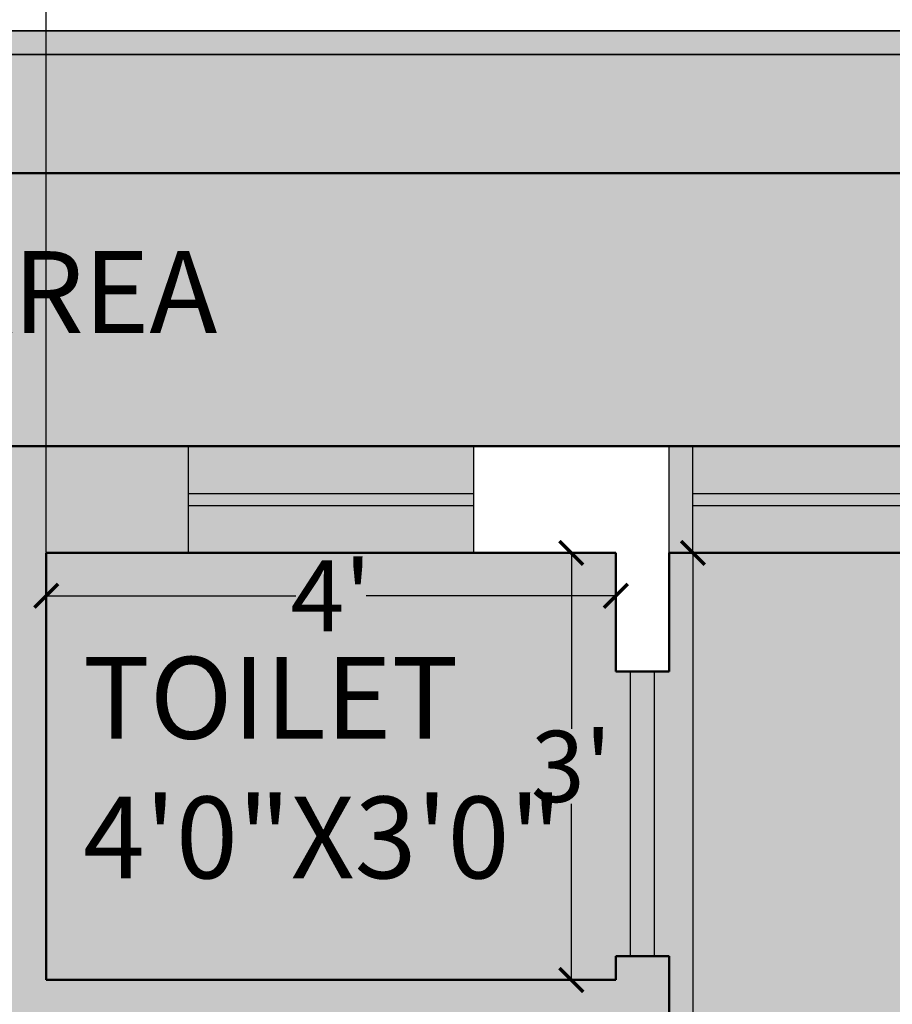
# Model space of a CAD drawing. Units: inches. Extents: x 528 to 2620, y -1066 to 798.
# Tile 17 of 41: x 776 to 850, y 672 to 755. Entities that reach past the tile are written whole.
import ezdxf

# ---------------------------------------------------------------- set-up
doc = ezdxf.new("R2010")
doc.units = ezdxf.units.IN
doc.header["$MEASUREMENT"] = 0
for name, color, linetype, lineweight in [('A-ANNO-DIMS', 2, 'Continuous', 18), ('A-AREA-IDEN', 7, 'Continuous', 18), ('A-Door', 2, 'Continuous', 25), ('A-GLAZ', 3, 'Continuous', 25), ('A-WALL', 7, 'Continuous', 50), ('A-WALL-PATT', 8, 'Continuous', 13), ('C-PROP', 5, 'Continuous', 35)]:
    doc.layers.add(name, color=color, linetype=linetype, lineweight=lineweight)
doc.styles.get("Standard").update_dxf_attribs({"font": 'arial.ttf'})
doc.dimstyles.get("Standard").update_dxf_attribs({"dimtxt": 6, "dimasz": 2, "dimexe": 0.18, "dimexo": 0.0625, "dimgap": 0.09, "dimtad": 0, "dimtih": 1, "dimtoh": 1, "dimdec": 1, "dimzin": 0, "dimdsep": 46, "dimlunit": 3, "dimtxsty": 'Standard', "dimblk": 'ARCHTICK', "dimcen": 0.09, "dimadec": 0, "dimazin": 0, "dimtfac": 1, "dimtdec": 1, "dimtofl": 0, "dimtmove": 0, "dimatfit": 3, "dimfxl": 1, "dimtolj": 1, "dimtzin": 0, "dimarcsym": 0})

# ---------------------------------------------------------------- blocks, each defined once
blk = doc.blocks.new('_ArchTick')
at = {"color": 0, "linetype": 'ByBlock', "const_width": 0.15}
blk.add_lwpolyline([(-0.5, -0.5), (0.5, 0.5)], dxfattribs=at)
blk = doc.blocks.new('*D11')
at = {"layer": 'A-ANNO-DIMS', "color": 0, "lineweight": -2, "transparency": 16777216}
for p, q in [((584.059, 753.985), (584.059, 794.007)), ((584.059, 793.827), (758.88, 793.827)), ((944.059, 793.827), (769.239, 793.827)), ((944.059, 753.985), (944.059, 794.007))]:
    blk.add_line(p, q, dxfattribs=at)
at = {"layer": 'Defpoints', "color": 0, "transparency": 16777216}
for p in [(944.059, 793.827), (584.059, 753.922), (944.059, 753.922)]:
    blk.add_point(p, dxfattribs=at)
at = {"layer": 'A-ANNO-DIMS', "color": 0, "lineweight": -2, "transparency": 16777216, "xscale": 2, "yscale": 2, "zscale": 2, "rotation": 180}
blk.add_blockref('_ArchTick', (584.059, 793.827), dxfattribs=at)
at = {"layer": 'A-ANNO-DIMS', "color": 0, "lineweight": -2, "transparency": 16777216, "xscale": 2, "yscale": 2, "zscale": 2}
blk.add_blockref('_ArchTick', (944.059, 793.827), dxfattribs=at)
at = {"layer": 'A-ANNO-DIMS', "color": 0, "transparency": 16777216, "insert": (764.059, 793.827), "char_height": 6, "attachment_point": 5}
blk.add_mtext("\\A1;30'", dxfattribs=at)
blk = doc.blocks.new('*D28')
at = {"layer": 'A-ANNO-DIMS', "color": 0, "lineweight": -2, "transparency": 16777216}
for p, q in [((833.059, 709.922), (833.059, 620.826)), ((833.122, 709.922), (833.239, 709.922)), ((833.059, 525.422), (833.059, 614.519)), ((833.102, 525.422), (832.879, 525.422))]:
    blk.add_line(p, q, dxfattribs=at)
at = {"layer": 'Defpoints', "color": 0, "transparency": 16777216}
for p in [(833.059, 709.922), (833.059, 709.922), (833.164, 525.422)]:
    blk.add_point(p, dxfattribs=at)
at = {"layer": 'A-ANNO-DIMS', "color": 0, "lineweight": -2, "transparency": 16777216, "xscale": 2, "yscale": 2, "zscale": 2}
for p, rotation in [((833.059, 709.922), 90), ((833.059, 525.422), 270)]:
    blk.add_blockref('_ArchTick', p, dxfattribs=dict(at, rotation=rotation))
at = {"layer": 'A-ANNO-DIMS', "color": 0, "transparency": 16777216, "insert": (833.059, 617.672), "char_height": 6, "attachment_point": 5}
blk.add_mtext('\\A1;15\'-4.5"', dxfattribs=at)
blk = doc.blocks.new('*D29')
at = {"layer": 'A-ANNO-DIMS', "color": 0, "lineweight": -2, "transparency": 16777216}
for p, q in [((822.67, 709.922), (822.995, 709.922)), ((822.815, 709.922), (822.815, 695.078)), ((822.815, 673.922), (822.815, 688.767)), ((822.67, 673.922), (822.995, 673.922))]:
    blk.add_line(p, q, dxfattribs=at)
at = {"layer": 'Defpoints', "color": 0, "transparency": 16777216}
for p in [(822.608, 709.922), (822.608, 673.922), (822.815, 673.922)]:
    blk.add_point(p, dxfattribs=at)
at = {"layer": 'A-ANNO-DIMS', "color": 0, "lineweight": -2, "transparency": 16777216, "xscale": 2, "yscale": 2, "zscale": 2}
for p, rotation in [((822.815, 709.922), 90), ((822.815, 673.922), 270)]:
    blk.add_blockref('_ArchTick', p, dxfattribs=dict(at, rotation=rotation))
at = {"layer": 'A-ANNO-DIMS', "color": 0, "transparency": 16777216, "insert": (822.815, 691.922), "char_height": 6, "attachment_point": 5}
blk.add_mtext("\\A1;3'", dxfattribs=at)
blk = doc.blocks.new('*D30')
at = {"layer": 'A-ANNO-DIMS', "color": 0, "lineweight": -2, "transparency": 16777216}
for p, q in [((778.559, 706.368), (778.559, 706.486)), ((778.559, 706.306), (799.588, 706.306)), ((826.559, 706.306), (805.531, 706.306)), ((826.559, 706.368), (826.559, 706.486))]:
    blk.add_line(p, q, dxfattribs=at)
at = {"layer": 'Defpoints', "color": 0, "transparency": 16777216}
for p in [(778.559, 706.306), (778.559, 706.306), (826.559, 706.306)]:
    blk.add_point(p, dxfattribs=at)
at = {"layer": 'A-ANNO-DIMS', "color": 0, "lineweight": -2, "transparency": 16777216, "xscale": 2, "yscale": 2, "zscale": 2, "rotation": 180}
blk.add_blockref('_ArchTick', (778.559, 706.306), dxfattribs=at)
at = {"layer": 'A-ANNO-DIMS', "color": 0, "lineweight": -2, "transparency": 16777216, "xscale": 2, "yscale": 2, "zscale": 2}
blk.add_blockref('_ArchTick', (826.559, 706.306), dxfattribs=at)
at = {"layer": 'A-ANNO-DIMS', "color": 0, "transparency": 16777216, "insert": (802.559, 706.306), "char_height": 6, "attachment_point": 5}
blk.add_mtext("\\A1;4'", dxfattribs=at)
blk = doc.blocks.new('WIN-1200')
for p, q in [((677.559, 718.922), (725.559, 718.922)), ((677.559, 709.922), (677.559, 718.922)), ((679.559, 709.922), (679.559, 718.922)), ((723.559, 718.922), (723.559, 709.922)), ((725.559, 718.922), (725.559, 709.922)), ((679.559, 714.922), (723.559, 714.922)), ((679.559, 713.922), (723.559, 713.922)), ((725.559, 709.922), (677.559, 709.922))]:
    blk.add_line(p, q)
blk = doc.blocks.new('WIN-600')
for p, q in [((790.559, 714.922), (814.559, 714.922)), ((790.559, 713.922), (814.559, 713.922))]:
    blk.add_line(p, q)
blk.add_lwpolyline([(790.559, 718.922), (814.559, 718.922), (814.559, 709.922), (790.559, 709.922)], close=True)
blk = doc.blocks.new('*D56')
at = {"layer": 'A-ANNO-DIMS', "color": 0, "lineweight": -2, "transparency": 16777216}
for p, q in [((774.059, 709.985), (774.059, 788.102)), ((774.059, 787.922), (778.559, 787.922)), ((778.559, 709.985), (778.559, 788.102)), ((778.559, 787.922), (780.559, 787.922))]:
    blk.add_line(p, q, dxfattribs=at)
at = {"layer": 'Defpoints', "color": 0, "transparency": 16777216}
for p in [(778.559, 787.922), (774.059, 709.922), (778.559, 709.922)]:
    blk.add_point(p, dxfattribs=at)
at = {"layer": 'A-ANNO-DIMS', "color": 0, "lineweight": -2, "transparency": 16777216, "xscale": 2, "yscale": 2, "zscale": 2, "rotation": 180}
blk.add_blockref('_ArchTick', (774.059, 787.922), dxfattribs=at)
at = {"layer": 'A-ANNO-DIMS', "color": 0, "lineweight": -2, "transparency": 16777216, "xscale": 2, "yscale": 2, "zscale": 2}
blk.add_blockref('_ArchTick', (778.559, 787.922), dxfattribs=at)
at = {"layer": 'A-ANNO-DIMS', "color": 0, "transparency": 16777216, "insert": (795.615, 787.922), "char_height": 6, "attachment_point": 5}
blk.add_mtext('\\A1;0\'-4 1/2"', dxfattribs=at)

msp = doc.modelspace()

# ---------------------------------------------------------------- hatches: boundary and pattern name
at = {"layer": 'A-Door', "transparency": 33554521}
h = msp.add_hatch(color=256, dxfattribs=at)
h.dxf.hatch_style = 1
h.paths.add_polyline_path([(829.809, 699.922), (827.809, 699.922), (827.809, 675.922), (829.809, 675.922)])
at = {"layer": 'A-WALL-PATT', "transparency": 33554687}
h = msp.add_hatch(color=256, dxfattribs=at)
h.dxf.hatch_style = 1
h.paths.add_polyline_path([(944.059, 753.922), (584.059, 753.922), (584.059, 208.922), (608.059, 208.922), (608.059, 210.922), (586.059, 210.922), (586.059, 751.922), (942.059, 751.922), (942.059, 210.922), (728.059, 210.922), (728.059, 208.922), (944.059, 208.922)])
h = msp.add_hatch(color=256, dxfattribs=at)
h.dxf.hatch_style = 1
h.paths.add_polyline_path([(942.059, 751.922), (586.059, 751.922), (586.059, 210.922), (608.059, 210.922), (608.059, 220.922), (596.059, 220.922), (596.059, 741.922), (932.059, 741.922), (932.059, 220.922), (770.059, 220.922), (728.059, 220.922), (728.059, 210.922), (942.059, 210.922)])
at = {"layer": 'A-WALL-PATT', "transparency": 33554475}
h = msp.add_hatch(color=256, dxfattribs=at)
h.dxf.hatch_style = 1
h.paths.add_polyline_path([(620.059, 718.922), (908.059, 718.922), (908.059, 268.922), (770.059, 268.922), (770.059, 220.922), (932.059, 220.922), (932.059, 741.922), (596.059, 741.922), (596.059, 391.422), (620.059, 391.422)])
at = {"layer": 'A-WALL-PATT', "transparency": 33554687}
h = msp.add_hatch(color=256, dxfattribs=at)
h.dxf.hatch_style = 1
h.paths.add_polyline_path([(861.059, 273.922), (817.059, 273.922), (817.059, 272.922), (861.059, 272.922)])
h.paths.add_polyline_path([(817.059, 277.922), (815.059, 277.922), (815.059, 268.922), (817.059, 268.922)])
h.paths.add_polyline_path([(908.059, 397.922), (899.059, 397.922), (899.059, 395.922), (908.059, 395.922)])
h.paths.add_polyline_path([(908.059, 443.922), (899.059, 443.922), (899.059, 441.922), (908.059, 441.922)])
h.paths.add_polyline_path([(904.059, 441.922), (903.059, 441.922), (903.059, 397.922), (904.059, 397.922)])
h.paths.add_polyline_path([(625.059, 561.422), (624.059, 561.422), (624.059, 537.422), (625.059, 537.422)])
h.paths.add_polyline_path([(648.747, 334.444), (720.045, 334.444), (720.045, 344.998), (648.747, 344.998)], flags=9)
h.paths.add_polyline_path([(819.733, 323.153), (880.328, 323.153), (880.328, 333.708), (819.733, 333.708)], flags=9)
h.paths.add_polyline_path([(779.898, 680.607), (821.764, 680.607), (821.764, 691.169), (779.898, 691.169)], flags=9)
h.paths.add_polyline_path([(779.876, 692.362), (817.138, 692.362), (817.138, 703.058), (779.876, 703.058)], flags=9)
h.paths.add_polyline_path([(799.994, 453.884), (860.589, 453.884), (860.589, 464.439), (799.994, 464.439)], flags=9)
h.paths.add_polyline_path([(650.866, 539.397), (708.781, 539.397), (708.781, 549.952), (650.866, 549.952)], flags=9)
h.paths.add_polyline_path([(788.504, 612.01), (849.099, 612.01), (849.099, 622.565), (788.504, 622.565)], flags=9)
h.paths.add_polyline_path([(639.539, 648.31), (700.134, 648.31), (700.134, 658.865), (639.539, 658.865)], flags=9)
h.paths.add_polyline_path([(648.913, 346.09), (747.706, 346.09), (747.706, 356.778), (648.913, 356.778)], flags=9)
h.paths.add_polyline_path([(676.857, 450.66), (746.735, 450.66), (746.735, 461.355), (676.857, 461.355)], flags=9)
h.paths.add_polyline_path([(819.711, 334.947), (865.526, 334.947), (865.526, 345.636), (819.711, 345.636)], flags=9)
h.paths.add_polyline_path([(806.298, 467.745), (874.047, 467.745), (874.047, 478.441), (806.298, 478.441)], flags=9)
h.paths.add_polyline_path([(653.235, 552.284), (690.497, 552.284), (690.497, 562.979), (653.235, 562.979)], flags=9)
h.paths.add_polyline_path([(789.903, 623.407), (843.208, 623.407), (843.208, 634.103), (789.903, 634.103)], flags=9)
h.paths.add_polyline_path([(639.773, 662.103), (693.077, 662.103), (693.077, 672.798), (639.773, 672.798)], flags=9)
h.paths.add_polyline_path([(801.587, 242.914), (846.334, 242.914), (846.334, 253.603), (801.587, 253.603)], flags=9)
h.paths.add_polyline_path([(925.362, 593.982), (925.362, 674.057), (914.673, 674.057), (914.673, 593.982)], flags=9)
h.paths.add_polyline_path([(612.559, 593.982), (612.559, 674.057), (601.871, 674.057), (601.871, 593.982)], flags=9)
h.paths.add_polyline_path([(723.31, 726.564), (803.385, 726.564), (803.385, 737.252), (723.31, 737.252)], flags=9)
at = {"layer": 'A-WALL-PATT', "transparency": 33554521}
h = msp.add_hatch(color=256, dxfattribs=at)
h.dxf.hatch_style = 1
h.paths.add_polyline_path([(629.059, 709.922), (677.559, 709.922), (677.559, 718.922), (620.059, 718.922), (620.059, 667.922), (629.059, 667.922)])
h.paths.add_polyline_path([(790.559, 718.922), (725.559, 718.922), (725.559, 709.922), (774.059, 709.922), (774.059, 577.922), (768.481, 577.922), (768.559, 573.422), (774.059, 573.422), (774.059, 567.422), (778.559, 567.422), (778.559, 669.422), (831.059, 669.422), (831.059, 675.922), (826.559, 675.922), (826.559, 673.922), (778.559, 673.922), (778.559, 709.922), (790.559, 709.922)])
h.paths.add_polyline_path([(908.059, 718.922), (879.059, 718.922), (879.059, 709.922), (899.059, 709.922), (899.059, 641.672), (908.059, 641.672)])
h.paths.add_polyline_path([(629.059, 619.922), (620.059, 619.922), (620.059, 561.422), (629.059, 561.422), (629.059, 573.422), (724.059, 573.422), (724.059, 569.422), (728.559, 569.422), (728.559, 577.922), (629.059, 577.922)])
h.paths.add_polyline_path([(779.059, 391.422), (779.059, 400.422), (770.059, 400.422), (764.059, 400.422), (764.059, 397.422), (764.059, 391.422), (770.059, 391.422), (770.059, 268.922), (815.059, 268.922), (815.059, 277.922), (779.059, 277.922), (779.059, 359.767)])
h.paths.add_polyline_path([(908.059, 395.922), (899.059, 395.922), (851.059, 395.922), (851.059, 391.422), (899.059, 391.422), (899.059, 277.922), (863.059, 277.922), (863.059, 268.922), (908.059, 268.922)])
h.paths.add_polyline_path([(908.059, 593.672), (899.059, 593.672), (899.059, 525.422), (778.559, 525.422), (778.559, 527.172), (774.059, 527.172), (774.059, 520.922), (899.059, 520.922), (899.059, 443.922), (908.059, 443.922)])
h.paths.add_polyline_path([(629.059, 520.922), (728.559, 520.922), (728.559, 545.422), (724.059, 545.422), (724.059, 525.422), (629.059, 525.422), (629.059, 537.422), (620.059, 537.422), (620.059, 484.672), (629.059, 484.672)])
h.paths.add_polyline_path([(629.059, 436.672), (620.059, 436.672), (620.059, 391.422), (648.559, 391.422), (648.559, 400.422), (629.059, 400.422)])
h.paths.add_polyline_path([(716.059, 397.422), (716.059, 400.422), (696.559, 400.422), (696.559, 391.422), (716.059, 391.422)])
at = {"layer": 'A-WALL-PATT', "transparency": 33554681}
h = msp.add_hatch(color=256, dxfattribs=at)
h.dxf.hatch_style = 1
h.paths.add_polyline_path([(629.059, 665.922), (625.059, 665.922), (625.059, 621.922), (629.059, 621.922)])
h.paths.add_polyline_path([(624.059, 665.922), (620.059, 665.922), (620.059, 621.922), (624.059, 621.922)])
h.paths.add_polyline_path([(723.559, 713.922), (679.559, 713.922), (679.559, 709.922), (723.559, 709.922)])
h.paths.add_polyline_path([(723.559, 718.922), (679.559, 718.922), (679.559, 714.922), (723.559, 714.922)])
h.paths.add_polyline_path([(814.559, 713.922), (790.559, 713.922), (790.559, 709.922), (814.559, 709.922)])
h.paths.add_polyline_path([(814.559, 718.922), (790.559, 718.922), (790.559, 714.922), (814.559, 714.922)])
h.paths.add_polyline_path([(877.059, 713.922), (833.059, 713.922), (833.059, 709.922), (877.059, 709.922)])
h.paths.add_polyline_path([(877.059, 718.922), (833.059, 718.922), (833.059, 714.922), (877.059, 714.922)])
h.paths.add_polyline_path([(908.059, 639.672), (904.059, 639.672), (904.059, 595.672), (908.059, 595.672)])
h.paths.add_polyline_path([(903.059, 639.672), (899.059, 639.672), (899.059, 595.672), (903.059, 595.672)])
h.paths.add_polyline_path([(908.059, 441.922), (904.059, 441.922), (904.059, 397.922), (908.059, 397.922)])
h.paths.add_polyline_path([(903.059, 441.922), (899.059, 441.922), (899.059, 397.922), (903.059, 397.922)])
h.paths.add_polyline_path([(861.059, 272.922), (817.059, 272.922), (817.059, 268.922), (861.059, 268.922)])
h.paths.add_polyline_path([(861.059, 277.922), (817.059, 277.922), (817.059, 273.922), (861.059, 273.922)])
h.paths.add_polyline_path([(694.559, 395.422), (650.559, 395.422), (650.559, 391.422), (694.559, 391.422)])
h.paths.add_polyline_path([(694.559, 400.422), (650.559, 400.422), (650.559, 396.422), (694.559, 396.422)])
h.paths.add_polyline_path([(629.059, 482.672), (625.059, 482.672), (625.059, 438.672), (629.059, 438.672)])
h.paths.add_polyline_path([(624.059, 482.672), (620.059, 482.672), (620.059, 438.672), (624.059, 438.672)])
h.paths.add_polyline_path([(629.059, 561.422), (625.059, 561.422), (625.059, 537.422), (629.059, 537.422)])
h.paths.add_polyline_path([(624.059, 561.422), (620.059, 561.422), (620.059, 537.422), (624.059, 537.422)])
h = msp.add_hatch(color=256, dxfattribs=at)
h.dxf.hatch_style = 1
h.paths.add_polyline_path([(625.059, 665.922), (624.059, 665.922), (624.059, 621.922), (625.059, 621.922)])
h.paths.add_polyline_path([(629.059, 667.922), (620.059, 667.922), (620.059, 665.922), (629.059, 665.922)])
h.paths.add_polyline_path([(629.059, 621.922), (620.059, 621.922), (620.059, 619.922), (629.059, 619.922)])
h.paths.add_polyline_path([(723.559, 714.922), (679.559, 714.922), (679.559, 713.922), (723.559, 713.922)])
h.paths.add_polyline_path([(725.559, 718.922), (723.559, 718.922), (723.559, 709.922), (725.559, 709.922)])
h.paths.add_polyline_path([(679.559, 718.922), (677.559, 718.922), (677.559, 709.922), (679.559, 709.922)])
h.paths.add_polyline_path([(814.559, 714.922), (790.559, 714.922), (790.559, 713.922), (814.559, 713.922)])
h.paths.add_polyline_path([(877.059, 714.922), (833.059, 714.922), (833.059, 713.922), (877.059, 713.922)])
h.paths.add_polyline_path([(879.059, 718.922), (877.059, 718.922), (877.059, 709.922), (879.059, 709.922)])
h.paths.add_polyline_path([(833.059, 718.922), (831.059, 718.922), (831.059, 709.922), (833.059, 709.922)])
h.paths.add_polyline_path([(650.559, 400.422), (648.559, 400.422), (648.559, 391.422), (650.559, 391.422)])
h.paths.add_polyline_path([(694.559, 396.422), (650.559, 396.422), (650.559, 395.422), (694.559, 395.422)])
h.paths.add_polyline_path([(696.559, 400.422), (694.559, 400.422), (694.559, 391.422), (696.559, 391.422)])
h.paths.add_polyline_path([(629.059, 438.672), (620.059, 438.672), (620.059, 436.672), (629.059, 436.672)])
h.paths.add_polyline_path([(629.059, 484.672), (620.059, 484.672), (620.059, 482.672), (629.059, 482.672)])
h.paths.add_polyline_path([(625.059, 482.672), (624.059, 482.672), (624.059, 438.672), (625.059, 438.672)])
at = {"layer": 'A-WALL-PATT', "transparency": 33554590}
h = msp.add_hatch(color=256, dxfattribs=at)
h.dxf.hatch_style = 1
h.paths.add_polyline_path([(774.059, 709.922), (629.059, 709.922), (629.059, 577.922), (728.559, 577.922), (728.559, 579.422), (728.559, 619.422), (730.309, 619.422), (730.309, 619.384, -0.401453), (768.559, 579.422), (768.559, 577.922), (774.059, 577.922)])
h.paths.add_polyline_path([(723.896, 686.058), (723.968, 686.064), (723.828, 686.128)], flags=0)
h.paths.add_polyline_path([(722.785, 642.699), (722.893, 642.756), (722.893, 684.992), (722.647, 685.244), (722.647, 685.82), (723.079, 686.262), (723.533, 686.262), (723.968, 686.064), (724.739, 686.128), (770.696, 686.128), (770.78, 686.14), (771.126, 686.266), (771.694, 686.094), (771.94, 685.478), (771.67, 684.904), (771.582, 684.871), (771.582, 642.782), (771.878, 642.514), (771.878, 641.921), (771.511, 641.462), (770.855, 641.462), (770.401, 641.833), (770.401, 641.551), (724.739, 641.551), (723.991, 641.705), (723.443, 641.414), (722.879, 641.585), (722.597, 642.142)], flags=16)
h.paths.add_polyline_path([(723.994, 641.704), (723.994, 641.707), (723.991, 641.705)], flags=0)
h.paths.add_polyline_path([(722.893, 642.732), (722.893, 684.992), (722.647, 685.244), (722.647, 685.82), (723.079, 686.262), (723.287, 686.262), (722.991, 686.172), (722.794, 685.971), (722.647, 685.68), (722.647, 685.434), (722.745, 685.143), (722.942, 684.942), (723.238, 684.807), (723.484, 684.807), (723.779, 684.897), (723.976, 685.098), (724.174, 685.488), (724.124, 685.635), (724.124, 685.249), (723.631, 684.746), (723.631, 642.961), (724.124, 642.514), (724.124, 641.887), (723.656, 641.462), (723.079, 641.462), (722.647, 641.904), (722.647, 642.48)], flags=0)
h.paths.add_polyline_path([(722.647, 642.29), (722.647, 642.044), (722.794, 641.753), (723.079, 641.462), (723.287, 641.462), (722.879, 641.585), (722.597, 642.142)], flags=0)
h.paths.add_polyline_path([(770.745, 686.128), (770.58, 686.128), (770.551, 686.057)], flags=0)
h.paths.add_polyline_path([(743.299, 645.288), (753.227, 659.398), (748.69, 663.75), (753.234, 668.538), (743.299, 682.458), (743.791, 682.592), (744.136, 682.681), (744.53, 682.928), (744.628, 683.084), (745.017, 683.327), (744.53, 684.069), (744.776, 684.158), (744.874, 684.315), (745.514, 684.404), (746.081, 684.651), (746.474, 684.651), (746.819, 684.807), (747.459, 685.031), (747.705, 685.143), (748.198, 685.277), (748.394, 685.523), (748.862, 685.523), (749.994, 686.128), (753.488, 676.03), (757.379, 680.153), (757.791, 679.758), (758.044, 680.645), (758.29, 681.227), (758.29, 682.055), (758.019, 682.592), (757.871, 683.174), (757.822, 683.778), (758.388, 684.069), (758.979, 684.203), (759.619, 684.158), (760.21, 683.957), (760.751, 683.666), (761.859, 683.666), (762.401, 683.957), (762.991, 684.114), (763.631, 684.114), (764.198, 683.957), (764.739, 683.666), (766.118, 683.666), (766.659, 683.957), (767.25, 684.158), (767.865, 684.203), (768.456, 684.069), (769.047, 683.778), (768.998, 683.174), (768.85, 682.592), (768.554, 682.055), (768.554, 681.227), (768.801, 680.645), (769.092, 679.75), (768.948, 678.832), (768.801, 678.228), (768.554, 677.646), (768.554, 676.818), (768.801, 676.237), (769.092, 675.341), (768.948, 674.424), (768.801, 673.82), (768.554, 673.283), (768.554, 672.41), (768.801, 671.873), (768.998, 671.291), (769.047, 670.642), (768.948, 670.016), (768.801, 669.411), (768.554, 668.874), (768.554, 668.002), (768.974, 667.239), (769.047, 666.279), (769.047, 665.563), (768.456, 665.316), (767.865, 665.16), (767.25, 665.16), (766.659, 665.361), (766.118, 665.697), (764.739, 665.697), (763.945, 665.204), (762.991, 665.204), (762.401, 665.361), (761.859, 665.697), (761.005, 665.697), (762.696, 664.086), (760.741, 662.027), (761.859, 662.027), (762.401, 662.318), (763.342, 662.548), (764.247, 662.318), (764.788, 662.027), (766.118, 662.027), (766.659, 662.318), (767.25, 662.519), (767.865, 662.564), (768.505, 662.43), (769.047, 662.116), (769.047, 661.4), (769.047, 660.796), (768.85, 660.214), (768.554, 659.677), (768.554, 658.849), (768.85, 658.267), (768.998, 657.663), (769.069, 656.749), (768.85, 655.851), (768.554, 655.269), (768.554, 654.441), (768.85, 653.859), (769.069, 652.961), (768.998, 652.046), (768.85, 651.442), (768.554, 650.905), (768.554, 650.032), (768.85, 649.495), (768.998, 648.914), (769.047, 648.265), (768.998, 647.638), (768.85, 647.034), (768.554, 646.497), (768.554, 645.624), (768.85, 645.087), (769.047, 644.55), (769.047, 643.901), (768.505, 643.655), (767.865, 643.521), (767.25, 643.521), (766.659, 643.722), (766.118, 644.058), (764.788, 644.058), (764.247, 643.722), (763.342, 643.492), (762.401, 643.722), (761.859, 644.058), (760.801, 644.058), (760.259, 643.722), (759.668, 643.521), (759.028, 643.521), (758.388, 643.655), (757.871, 643.901), (757.871, 644.55), (758.044, 645.087), (758.339, 645.624), (758.339, 646.497), (758.044, 647.034), (757.921, 647.638), (757.866, 648.059), (757.379, 647.593), (753.422, 651.773), (749.994, 641.618), (749.502, 641.708), (749.354, 641.954), (748.542, 642.446), (747.311, 642.939), (746.652, 642.939), (746.327, 643.185), (745.514, 643.565), (744.53, 643.655), (745.011, 644.4), (744.628, 644.639), (744.136, 644.886), (743.791, 645.132)], flags=0)
h.paths.add_polyline_path([(755.656, 654.933), (756.542, 654.687), (757.527, 654.329), (756.641, 654.575)], flags=0)
h.paths.add_polyline_path([(758.339, 649.204), (758.339, 648.712), (758.585, 644.304), (758.585, 648.802)], flags=0)
h.paths.add_polyline_path([(758.339, 649.294), (758.093, 649.697), (758.359, 649.165)], flags=0)
h.paths.add_polyline_path([(755.656, 672.79), (756.493, 673.037), (757.358, 673.351), (757.353, 673.358), (756.641, 673.149)], flags=0)
h.paths.add_polyline_path([(760.264, 639.641), (771.408, 639.641), (771.408, 624.039), (760.264, 624.039)], flags=16)
h.paths.add_polyline_path([(761.378, 638.526), (770.294, 638.526), (770.294, 625.153), (761.378, 625.153)], flags=0)
edge = h.paths.add_edge_path(flags=0)
edge.add_ellipse((765.836, 631.84), major_axis=(-2.245, 2.245), ratio=1, start_angle=-45, end_angle=45, ccw=False)
edge.add_ellipse((765.836, 631.84), major_axis=(-2.245, 2.245), ratio=1, start_angle=-135, end_angle=-45, ccw=False)
edge.add_ellipse((765.836, 631.84), major_axis=(-2.245, 2.245), ratio=1, start_angle=135, end_angle=-135, ccw=False)
edge.add_ellipse((765.836, 631.84), major_axis=(-2.245, 2.245), ratio=1, start_angle=45, end_angle=135, ccw=False)
h.paths.add_polyline_path([(758.585, 683.42), (758.585, 678.922), (758.373, 678.575), (758.339, 678.43), (758.093, 678.049), (758.339, 678.519), (758.339, 679.011)], flags=0)
h.paths.add_polyline_path([(760.264, 688.038), (760.264, 703.64), (771.408, 703.64), (771.408, 688.038)], flags=16)
h.paths.add_polyline_path([(770.401, 685.389), (770.401, 685.846), (770.855, 686.217), (771.511, 686.217), (771.878, 685.758), (771.878, 685.165), (771.582, 684.897), (771.582, 642.782), (771.878, 642.514), (771.878, 641.921), (771.511, 641.462), (770.855, 641.462), (770.401, 641.833), (770.401, 642.29)], flags=0)
h.paths.add_polyline_path([(770.532, 642.678), (771.052, 643.009), (771.67, 642.775), (771.94, 642.201), (771.694, 641.585), (771.126, 641.413), (770.551, 641.622), (770.347, 642.132)], flags=16)
h.paths.add_polyline_path([(761.378, 689.152), (761.378, 702.526), (770.294, 702.526), (770.294, 689.152)], flags=0)
edge = h.paths.add_edge_path(flags=0)
edge.add_ellipse((765.836, 695.839), major_axis=(2.245, 2.245), ratio=1, start_angle=405, end_angle=495, ccw=False)
edge.add_ellipse((765.836, 695.839), major_axis=(2.245, 2.245), ratio=1, start_angle=675, end_angle=765, ccw=False)
edge.add_ellipse((765.836, 695.839), major_axis=(2.245, 2.245), ratio=1, start_angle=585, end_angle=675, ccw=False)
edge.add_ellipse((765.836, 695.839), major_axis=(2.245, 2.245), ratio=1, start_angle=495, end_angle=585, ccw=False)
h.paths.add_polyline_path([(770.696, 684.897), (770.942, 684.74), (771.41, 684.74), (771.73, 685.031), (771.878, 685.344), (771.878, 685.635), (771.694, 686.094), (771.582, 686.128), (771.878, 685.758), (771.878, 685.165), (771.41, 684.74), (770.849, 684.74)], flags=0)
h.paths.add_polyline_path([(899.059, 709.922), (831.059, 709.922), (831.059, 699.922), (829.809, 699.922), (829.809, 675.922), (831.059, 675.922), (831.059, 669.422), (778.559, 669.422), (778.559, 567.172), (780.059, 567.172), (820.059, 567.172), (820.059, 565.422), (820.021, 565.422, -0.401453), (780.059, 527.172), (778.559, 527.172), (778.559, 525.422), (899.059, 525.422)])
h.paths.add_polyline_path([(849.197, 636.014), (849.269, 636.02), (849.129, 636.084)], flags=0)
h.paths.add_polyline_path([(848.193, 634.948), (847.947, 635.2), (847.947, 635.776), (848.379, 636.218), (848.833, 636.218), (849.269, 636.02), (850.039, 636.084), (895.996, 636.084), (896.081, 636.096), (896.426, 636.222), (896.995, 636.05), (897.241, 635.434), (896.97, 634.86), (896.883, 634.827), (896.883, 592.738), (897.178, 592.47), (897.178, 591.877), (896.811, 591.418), (896.155, 591.418), (895.701, 591.789), (895.701, 591.507), (850.039, 591.507), (849.292, 591.661), (848.744, 591.37), (848.18, 591.541), (847.897, 592.098), (848.086, 592.655), (848.193, 592.712)], flags=16)
h.paths.add_polyline_path([(849.294, 591.66), (849.295, 591.663), (849.292, 591.661)], flags=16)
h.paths.add_polyline_path([(848.193, 634.948), (847.947, 635.2), (847.947, 635.776), (848.379, 636.218), (848.587, 636.218), (848.292, 636.128), (848.095, 635.927), (847.947, 635.636), (847.947, 635.39), (848.046, 635.099), (848.243, 634.897), (848.538, 634.763), (848.784, 634.763), (849.079, 634.853), (849.276, 635.054), (849.474, 635.444), (849.424, 635.591), (849.424, 635.205), (848.932, 634.702), (848.932, 592.917), (849.424, 592.47), (849.424, 591.843), (848.956, 591.418), (848.379, 591.418), (847.947, 591.86), (847.947, 592.436), (848.193, 592.688)], flags=0)
h.paths.add_polyline_path([(847.947, 592.246), (847.947, 592), (848.095, 591.709), (848.379, 591.418), (848.587, 591.418), (848.18, 591.541), (847.897, 592.098)], flags=16)
h.paths.add_polyline_path([(896.046, 636.084), (895.88, 636.084), (895.852, 636.013)], flags=0)
h.paths.add_polyline_path([(868.599, 632.414), (869.092, 632.548), (869.436, 632.637), (869.83, 632.884), (869.929, 633.04), (870.318, 633.283), (869.83, 634.025), (870.076, 634.114), (870.175, 634.271), (870.815, 634.36), (871.381, 634.607), (871.775, 634.607), (872.119, 634.763), (872.759, 634.987), (873.006, 635.099), (873.498, 635.233), (873.695, 635.479), (874.163, 635.479), (875.295, 636.084), (878.788, 625.986), (882.679, 630.109), (883.091, 629.714), (883.344, 630.601), (883.59, 631.183), (883.59, 632.011), (883.319, 632.548), (883.172, 633.13), (883.123, 633.734), (883.689, 634.025), (884.279, 634.159), (884.919, 634.114), (885.51, 633.913), (886.052, 633.622), (887.159, 633.622), (887.701, 633.913), (888.292, 634.07), (888.932, 634.07), (889.498, 633.913), (890.039, 633.622), (891.418, 633.622), (891.959, 633.913), (892.55, 634.114), (893.166, 634.159), (893.756, 634.025), (894.347, 633.734), (894.298, 633.13), (894.15, 632.548), (893.855, 632.011), (893.855, 631.183), (894.101, 630.601), (894.393, 629.706), (894.249, 628.788), (894.101, 628.184), (893.855, 627.602), (893.855, 626.774), (894.101, 626.193), (894.393, 625.297), (894.249, 624.38), (894.101, 623.776), (893.855, 623.239), (893.855, 622.366), (894.101, 621.829), (894.298, 621.247), (894.347, 620.598), (894.249, 619.972), (894.101, 619.367), (893.855, 618.83), (893.855, 617.958), (894.274, 617.195), (894.347, 616.235), (894.347, 615.518), (893.756, 615.272), (893.166, 615.116), (892.55, 615.116), (891.959, 615.317), (891.418, 615.653), (890.039, 615.653), (889.245, 615.16), (888.292, 615.16), (887.701, 615.317), (887.159, 615.653), (886.305, 615.653), (887.996, 614.042), (886.041, 611.983), (887.159, 611.983), (887.701, 612.274), (888.642, 612.504), (889.547, 612.274), (890.089, 611.983), (891.418, 611.983), (891.959, 612.274), (892.55, 612.475), (893.166, 612.52), (893.806, 612.386), (894.347, 612.072), (894.347, 611.356), (894.347, 610.752), (894.15, 610.17), (893.855, 609.633), (893.855, 608.805), (894.15, 608.223), (894.298, 607.619), (894.37, 606.705), (894.15, 605.807), (893.855, 605.225), (893.855, 604.397), (894.15, 603.815), (894.37, 602.917), (894.298, 602.002), (894.15, 601.398), (893.855, 600.861), (893.855, 599.988), (894.15, 599.451), (894.298, 598.87), (894.347, 598.221), (894.298, 597.594), (894.15, 596.99), (893.855, 596.453), (893.855, 595.58), (894.15, 595.043), (894.347, 594.506), (894.347, 593.857), (893.806, 593.611), (893.166, 593.477), (892.55, 593.477), (891.959, 593.678), (891.418, 594.014), (890.089, 594.014), (889.547, 593.678), (888.642, 593.448), (887.701, 593.678), (887.159, 594.014), (886.101, 594.014), (885.559, 593.678), (884.969, 593.477), (884.329, 593.477), (883.689, 593.611), (883.172, 593.857), (883.172, 594.506), (883.344, 595.043), (883.639, 595.58), (883.639, 596.453), (883.344, 596.99), (883.221, 597.594), (883.167, 598.015), (882.679, 597.549), (878.722, 601.729), (875.295, 591.574), (874.803, 591.664), (874.655, 591.91), (873.843, 592.402), (872.612, 592.895), (871.952, 592.895), (871.627, 593.141), (870.815, 593.521), (869.83, 593.611), (870.311, 594.356), (869.929, 594.595), (869.436, 594.842), (869.092, 595.088), (868.599, 595.244), (878.528, 609.354), (873.99, 613.706), (878.535, 618.494)], flags=0)
h.paths.add_polyline_path([(880.956, 622.746), (881.793, 622.993), (882.659, 623.307), (882.654, 623.314), (881.941, 623.104)], flags=0)
h.paths.add_polyline_path([(880.956, 604.889), (881.843, 604.643), (882.827, 604.285), (881.941, 604.531)], flags=16)
h.paths.add_polyline_path([(883.393, 628.005), (883.639, 628.475), (883.639, 628.967), (883.886, 633.376), (883.886, 628.878), (883.674, 628.531), (883.639, 628.386)], flags=0)
h.paths.add_polyline_path([(883.639, 599.16), (883.639, 598.668), (883.886, 594.26), (883.886, 598.758)], flags=16)
h.paths.add_polyline_path([(883.639, 599.25), (883.393, 599.653), (883.659, 599.121)], flags=16)
h.paths.add_polyline_path([(885.564, 637.994), (885.564, 653.596), (896.709, 653.596), (896.709, 637.994)], flags=16)
h.paths.add_polyline_path([(885.564, 589.597), (896.709, 589.597), (896.709, 573.995), (885.564, 573.995)], flags=16)
h.paths.add_polyline_path([(886.679, 639.108), (886.679, 652.482), (895.594, 652.482), (895.594, 639.108)], flags=0)
h.paths.add_polyline_path([(886.679, 588.482), (895.594, 588.482), (895.594, 575.109), (886.679, 575.109)], flags=0)
edge = h.paths.add_edge_path(flags=0)
edge.add_ellipse((891.136, 645.795), major_axis=(2.245, 2.245), ratio=1, start_angle=405, end_angle=495, ccw=False)
edge.add_ellipse((891.136, 645.795), major_axis=(2.245, 2.245), ratio=1, start_angle=675, end_angle=765, ccw=False)
edge.add_ellipse((891.136, 645.795), major_axis=(2.245, 2.245), ratio=1, start_angle=585, end_angle=675, ccw=False)
edge.add_ellipse((891.136, 645.795), major_axis=(2.245, 2.245), ratio=1, start_angle=495, end_angle=585, ccw=False)
edge = h.paths.add_edge_path(flags=0)
edge.add_ellipse((891.136, 581.796), major_axis=(-2.245, 2.245), ratio=1, start_angle=-45, end_angle=45, ccw=False)
edge.add_ellipse((891.136, 581.796), major_axis=(-2.245, 2.245), ratio=1, start_angle=-135, end_angle=-45, ccw=False)
edge.add_ellipse((891.136, 581.796), major_axis=(-2.245, 2.245), ratio=1, start_angle=135, end_angle=-135, ccw=False)
edge.add_ellipse((891.136, 581.796), major_axis=(-2.245, 2.245), ratio=1, start_angle=45, end_angle=135, ccw=False)
h.paths.add_polyline_path([(895.701, 635.345), (895.701, 635.802), (896.155, 636.173), (896.811, 636.173), (897.178, 635.714), (897.178, 635.121), (896.883, 634.853), (896.883, 592.738), (897.178, 592.47), (897.178, 591.877), (896.811, 591.418), (896.155, 591.418), (895.701, 591.789), (895.701, 592.246)], flags=0)
h.paths.add_polyline_path([(895.996, 634.853), (896.243, 634.696), (896.71, 634.696), (897.03, 634.987), (897.178, 635.3), (897.178, 635.591), (896.995, 636.05), (896.883, 636.084), (897.178, 635.714), (897.178, 635.121), (896.71, 634.696), (896.15, 634.696)], flags=0)
h.paths.add_polyline_path([(895.832, 592.634), (896.353, 592.965), (896.97, 592.731), (897.241, 592.157), (896.995, 591.541), (896.426, 591.369), (895.852, 591.578), (895.648, 592.088)], flags=16)
h.paths.add_polyline_path([(725.255, 569.422), (724.059, 569.422), (724.059, 573.422), (629.059, 573.422), (629.059, 525.422), (724.059, 525.422), (724.059, 545.422), (725.255, 545.422)])
h.paths.add_polyline_path([(820.021, 565.422), (780.059, 565.422), (780.059, 567.172), (774.059, 567.172), (774.059, 567.422), (774.059, 573.422), (768.559, 573.422), (768.481, 577.922), (768.559, 577.922), (768.559, 579.422, 0.401453), (730.309, 619.384), (730.309, 579.422), (728.559, 579.422), (728.559, 573.422), (728.559, 569.422), (727.255, 569.422), (727.255, 545.422), (728.559, 545.422), (728.559, 520.922), (665.059, 520.922), (665.059, 436.422), (716.059, 436.422), (716.059, 421.422), (717.809, 421.422), (717.809, 421.358, -0.392996), (740.059, 397.422, -0.392996), (762.309, 421.358), (762.309, 421.422), (764.059, 421.422), (764.059, 400.422), (770.059, 400.422), (779.059, 400.422), (779.059, 391.422), (779.059, 359.767), (795.432, 359.767), (795.432, 294.295), (893.669, 294.295), (893.669, 277.922), (899.059, 277.922), (899.059, 391.422), (851.059, 391.422), (851.059, 395.922), (899.059, 395.922), (899.059, 443.922), (899.059, 520.922), (774.059, 520.922), (774.059, 527.172), (778.559, 527.172), (780.059, 527.172, 0.401453)])
h.paths.add_polyline_path([(774.059, 519.657), (842.122, 519.657), (842.122, 505.072), (788.644, 505.072), (788.644, 474.079), (788.644, 470.433, -0.883215), (779.529, 456.663), (774.971, 456.663, -0.414214), (774.059, 457.575)], flags=16)
h.paths.add_polyline_path([(775.883, 517.834), (840.299, 517.834), (840.299, 514.188), (788.644, 514.188), (788.644, 484.41), (779.529, 484.41), (779.529, 474.079), (775.883, 474.079)], flags=0)
h.paths.add_polyline_path([(706.7, 501.564, -0.254069), (706.7, 493.021), (698.31, 492.555), (698.31, 502.031)], flags=16)
h.paths.add_polyline_path([(691.334, 515.692), (691.8, 507.301), (682.325, 507.301), (682.791, 515.692, -0.254069)], flags=16)
h.paths.add_polyline_path([(695.485, 504.685), (695.485, 479.416), (678.64, 479.416), (678.64, 504.685)], flags=16)
h.paths.add_polyline_path([(706.7, 489.602, -0.254069), (706.7, 481.058), (698.31, 480.592), (698.31, 490.068)], flags=16)
h.paths.add_polyline_path([(675.815, 502.031), (675.815, 492.555), (667.425, 493.021, -0.254069), (667.425, 501.564)], flags=16)
h.paths.add_polyline_path([(691.8, 476.8), (691.334, 468.409, -0.254069), (682.791, 468.409), (682.325, 476.8)], flags=16)
h.paths.add_polyline_path([(675.815, 490.068), (675.815, 480.592), (667.425, 481.058, -0.254069), (667.425, 489.602)], flags=16)
h.paths.add_polyline_path([(764.059, 397.422), (762.309, 397.422), (762.309, 421.358, 0.392996), (740.059, 397.422, 0.392996), (717.809, 421.358), (717.809, 397.422), (716.059, 397.422), (716.059, 391.422), (716.059, 385.422), (764.059, 385.422), (764.059, 391.422)], flags=17)
h.paths.add_polyline_path([(716.059, 436.422), (705.859, 436.422), (705.859, 418.422), (716.059, 418.422), (716.059, 421.422)], flags=17)
h.paths.add_polyline_path([(716.059, 418.422), (705.859, 418.422), (705.859, 400.422), (716.059, 400.422)], flags=17)
h.paths.add_polyline_path([(705.859, 418.422), (695.659, 418.422), (695.659, 400.422), (696.559, 400.422), (705.859, 400.422)], flags=17)
h.paths.add_polyline_path([(705.859, 436.422), (695.659, 436.422), (695.659, 418.422), (705.859, 418.422)], flags=17)
h.paths.add_polyline_path([(695.659, 418.422), (685.459, 418.422), (685.459, 400.422), (695.659, 400.422)], flags=17)
h.paths.add_polyline_path([(695.659, 436.422), (685.459, 436.422), (685.459, 418.422), (695.659, 418.422)], flags=17)
h.paths.add_polyline_path([(685.459, 418.422), (675.259, 418.422), (675.259, 400.422), (685.459, 400.422)], flags=17)
h.paths.add_polyline_path([(685.459, 436.422), (675.259, 436.422), (675.259, 418.422), (685.459, 418.422)], flags=17)
h.paths.add_polyline_path([(675.259, 436.422), (665.059, 436.422), (665.059, 418.422), (675.259, 418.422)])
h.paths.add_polyline_path([(675.259, 418.422), (665.059, 418.422), (665.059, 400.422), (675.259, 400.422)])
h.paths.add_polyline_path([(665.059, 418.422), (646.967, 418.422), (646.991, 436.422), (629.059, 436.422), (629.059, 400.422), (665.059, 400.422)])
h.paths.add_polyline_path([(665.059, 436.422), (646.991, 436.422), (646.967, 418.422), (665.059, 418.422)], flags=17)
h.paths.add_polyline_path([(647.005, 446.622), (629.059, 446.622), (629.059, 436.672), (629.059, 436.422), (646.991, 436.422)])
h.paths.add_polyline_path([(665.059, 446.622), (647.005, 446.622), (646.991, 436.422), (665.059, 436.422)])
h.paths.add_polyline_path([(647.019, 456.822), (629.059, 456.822), (629.059, 446.622), (647.005, 446.622)])
h.paths.add_polyline_path([(665.059, 456.822), (647.019, 456.822), (647.005, 446.622), (665.059, 446.622)])
h.paths.add_polyline_path([(647.032, 467.022), (629.059, 467.022), (629.059, 456.822), (647.019, 456.822)])
h.paths.add_polyline_path([(665.059, 467.022), (647.032, 467.022), (647.019, 456.822), (665.059, 456.822)])
h.paths.add_polyline_path([(665.059, 477.222), (647.046, 477.222), (647.032, 467.022), (665.059, 467.022)])
h.paths.add_polyline_path([(647.046, 477.222), (629.059, 477.222), (629.059, 467.022), (647.032, 467.022)])
h.paths.add_polyline_path([(647.059, 487.222), (629.059, 487.222), (629.059, 477.222), (647.046, 477.222), (647.048, 479.019), (645.53, 483.246), (640.877, 480.371)])
h.paths.add_polyline_path([(665.059, 520.922), (629.059, 520.922), (629.059, 487.222), (647.059, 487.222), (665.059, 487.222)])
h.paths.add_polyline_path([(665.059, 487.222), (647.059, 487.222), (653.224, 480.355), (648.578, 483.242), (647.048, 479.019), (647.046, 477.222), (665.059, 477.222)])
at = {"layer": 'A-WALL-PATT', "transparency": 33554567}
h = msp.add_hatch(color=256, dxfattribs=at)
h.dxf.hatch_style = 1
h.paths.add_polyline_path([(827.809, 699.922), (826.559, 699.922), (826.559, 709.922), (778.559, 709.922), (778.559, 673.922), (826.559, 673.922), (826.559, 675.922), (827.809, 675.922)])
h.paths.add_polyline_path([(779.898, 680.607), (821.764, 680.607), (821.764, 691.169), (779.898, 691.169)], flags=24)
h.paths.add_polyline_path([(779.876, 692.362), (817.138, 692.362), (817.138, 703.058), (779.876, 703.058)], flags=24)

# ---------------------------------------------------------------- linework, layer by layer
at = {"layer": 'A-Door'}
msp.add_lwpolyline([(829.809, 675.922), (827.809, 675.922), (827.809, 699.922), (829.809, 699.922)], close=True, dxfattribs=at)
at = {"layer": 'A-WALL'}
for p, q in [((932.059, 741.922), (596.059, 741.922)), ((908.059, 718.922), (620.059, 718.922)), ((825.559, 709.922), (778.559, 709.922)), ((778.559, 709.922), (778.559, 673.922)), ((826.559, 709.922), (778.559, 709.922)), ((826.559, 709.922), (826.559, 699.922)), ((899.059, 709.922), (831.059, 709.922)), ((899.059, 709.922), (831.059, 709.922)), ((831.059, 709.922), (831.059, 699.922)), ((826.559, 699.922), (831.059, 699.922)), ((826.559, 675.922), (831.059, 675.922)), ((826.559, 675.922), (826.559, 673.922)), ((831.059, 675.922), (831.059, 669.422)), ((826.559, 673.922), (778.559, 673.922))]:
    msp.add_line(p, q, dxfattribs=at)
at = {"layer": 'C-PROP'}
for points in [[(728.059, 208.922), (944.059, 208.922), (944.059, 753.922), (584.059, 753.922), (584.059, 208.922), (608.059, 208.922)], [(728.059, 210.922), (942.059, 210.922), (942.059, 751.922), (586.059, 751.922), (586.059, 210.922), (608.059, 210.922)]]:
    msp.add_lwpolyline(points, dxfattribs=at)
msp.add_lwpolyline([(596.059, 741.922), (596.059, 220.922), (932.059, 220.922), (932.059, 741.922)], close=True, dxfattribs=at)

# ---------------------------------------------------------------- block references
at = {"layer": 'A-GLAZ'}
for name, p in [('WIN-600', (0, 0)), ('WIN-1200', (153.5, 0))]:
    msp.add_blockref(name, p, dxfattribs=at)

# ---------------------------------------------------------------- texts
at = {"layer": 'A-AREA-IDEN'}
for s, height, p in [('SET BACK AREA', 6.89074, (725.091, 728.463)), ('TOILET', 6.8907, (781.658, 694.262)), ('4\'0"X3\'0"', 6.8907, (781.658, 682.49))]:
    msp.add_text(s, height=height, dxfattribs=at).set_placement(p)

# ---------------------------------------------------------------- dimensions: what is measured, and where the dimension line sits
at = {"layer": 'A-ANNO-DIMS'}
for base, p1, p2, override, picture, middle in [((944.059, 793.827), (584.059, 753.922), (944.059, 753.922), {"dimclrd": 0, "dimclre": 0, "dimclrt": 0}, '*D11', (764.059, 793.827)), ((778.559, 787.922), (774.059, 709.922), (778.559, 709.922), {"dimdec": 1, "dimlfac": 1, "dimrnd": 0, "dimzin": 1, "dimdsep": 46, "dimlunit": 4, "dimfrac": 2}, '*D56', (795.615, 787.922)), ((778.559, 706.306), (826.559, 706.306), (778.559, 706.306), {"dimclrd": 0, "dimclre": 0, "dimclrt": 0}, '*D30', (802.559, 706.306))]:
    dim = msp.add_linear_dim(base=base, p1=p1, p2=p2, dimstyle='Standard', override=override, dxfattribs=at)
    dim.commit()
    dim.dimension.update_dxf_attribs({"geometry": picture, "text_midpoint": middle})
for base, p1, p2, picture, middle in [((833.059, 709.922), (833.164, 525.422), (833.059, 709.922), '*D28', (833.059, 617.672)), ((822.815, 673.922), (822.608, 709.922), (822.608, 673.922), '*D29', (822.815, 691.922))]:
    dim = msp.add_linear_dim(base=base, p1=p1, p2=p2, angle=90, dimstyle='Standard', override={"dimclrd": 0, "dimclre": 0, "dimclrt": 0}, dxfattribs=at)
    dim.commit()
    dim.dimension.update_dxf_attribs({"geometry": picture, "text_midpoint": middle})

doc.saveas('drawing.dxf')
